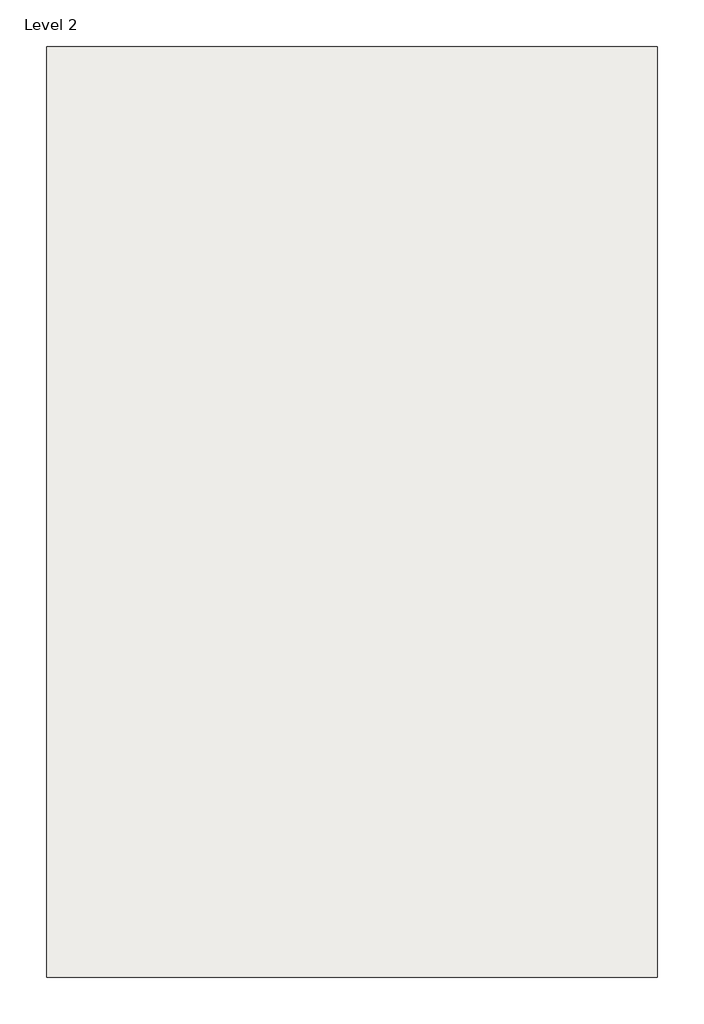
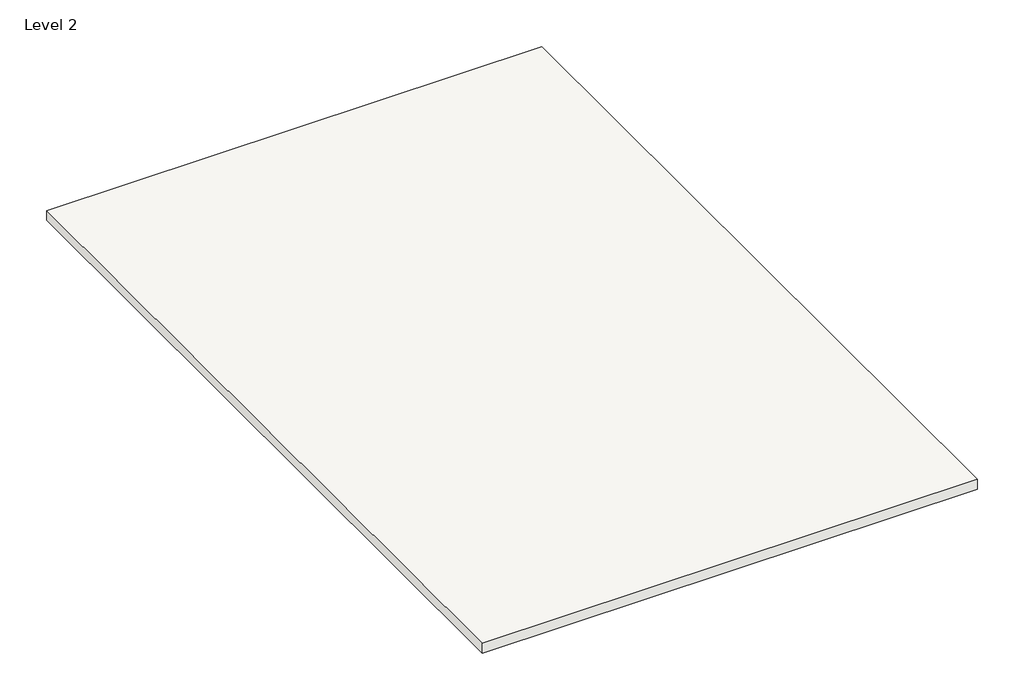
# One storey: 1 roof.
"""IFC4 building model written with IfcOpenShell, lengths in millimetres."""

from ifc_helpers import new_model, si_unit, frame, origin, place, context, project, spatial, polyline, outline, extrude, element, save

model = new_model("IFC4")

# Units and contexts
model_context = context("Model", 3, world=origin())
ifc_project = project(units=[si_unit("LENGTHUNIT", "METRE", prefix="MILLI")], contexts=[model_context])

# Site, building, storey
site = spatial("IfcSite", under=ifc_project)
building = spatial("IfcBuilding", under=site)
storey = spatial("IfcBuildingStorey", under=building, Name="Level 2", Elevation=3048.0)

# Roof
placement = place(None, origin())
element("IfcRoof", 1, ObjectType="Generic - 12\"", at=placement, inside=storey, context=model_context, shape_type="SweptSolid", body=[
    extrude(outline(polyline([(-15067.7446525, 12659.3002171), (-437.3446525, 12659.3002171), (-437.3446525, -9641.8997829), (-15067.7446525, -9641.8997829), (-15067.7446525, 12659.3002171)])), frame((0.0, 0.0, 3048.0), z_axis=(0.0, 0.0, 1.0), x_axis=(1.0, 0.0, 0.0)), (0.0, 0.0, 1.0), 304.8),
])

save(model, "model.ifc")

# Revit data of these elements
# Type "Generic - 12\""
#   Assembly Code = "B1020"
#   Layers, outside or top first: 1' - 0" "Brick, Soldier Course" (function 1)
# Element 1 (IfcRoof, "Generic - 12\"")
#   built-in parameter 1001705 = 11 (stored number, unit not read)
#   built-in parameter 1001710 = 33615
#   Phase Created = New Construction
#   Materials on its faces: "Brick, Soldier Course"
# Materials
#   "Brick, Soldier Course": class "Masonry", colour RGB 170 98 104, transparency 0, Description = "Common brick soldier coursed", Cost = 0
